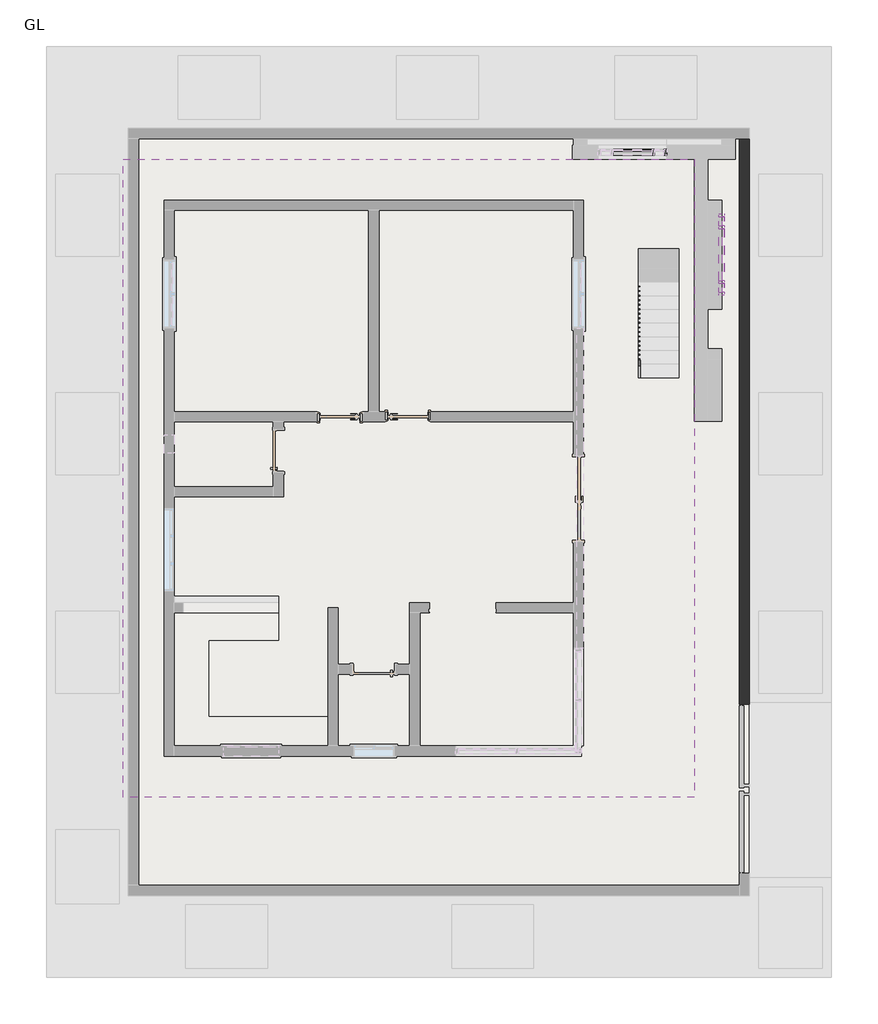
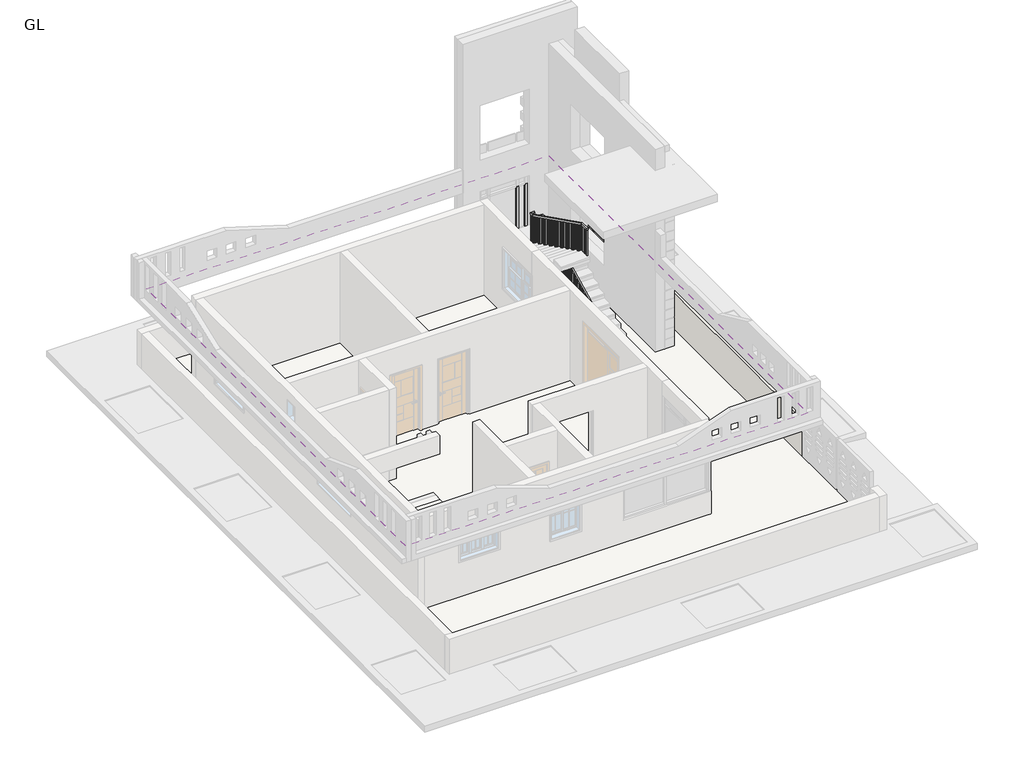
# One storey, part 3 of 4: 13 members, 3 plates, 2 slabs, 1 railing, 1 roof, 1 wall.
"""IFC4 building model written with IfcOpenShell, lengths in millimetres."""

from ifc_helpers import new_model, si_unit, frame, origin, origin_with_axes, place, context, project, spatial, polyline, outline, extrude, faceted_brep, transform, mapped, element, save
from components import member_e8ffc670, member_0c289f97, member_3782c11a, member_285512ba, member_6b401d40, member_96c05505, member_4491d118, member_82905deb, system_panel_glazed_d23cfa45, system_panel_glazed_ccd8c114, system_panel_glazed_e991d7fc

model = new_model("IFC4")

# Units and contexts
model_context = context("Model", 3, world=origin())
ifc_project = project(units=[si_unit("LENGTHUNIT", "METRE", prefix="MILLI")], contexts=[model_context])

# Site, building, storey
site = spatial("IfcSite", under=ifc_project)
building = spatial("IfcBuilding", under=site)
storey = spatial("IfcBuildingStorey", under=building, Name="GL", Elevation=0.0)

# Members
placement = place(None, origin())
member_shape = member_e8ffc670(model_context)
element("IfcMember", 1, ObjectType="Rectangular Mullion : 2.5\" x 5\" rectangular", at=placement, inside=storey, context=model_context, shape_type="MappedRepresentation", body=[
    mapped(member_shape, transform((872.7722402, 10698.1342801, 2741.3131867), x_axis=(0.0, 0.0, 1.0), y_axis=(1.0, 0.0, 0.0), z_axis=(0.0, 1.0, 0.0))),
])
member_2_shape = member_0c289f97(model_context)
element("IfcMember", 2, ObjectType="Rectangular Mullion : 2.5\" x 5\" rectangular", at=placement, inside=storey, context=model_context, shape_type="MappedRepresentation", body=[
    mapped(member_2_shape, transform((872.7722402, 8943.6292801, 2741.3131867), x_axis=(0.0, -1.0, 0.0), y_axis=(1.0, 0.0, 0.0), z_axis=(0.0, 0.0, 1.0))),
])
member_3_shape = member_3782c11a(model_context)
element("IfcMember", 3, ObjectType="Rectangular Mullion : 2.5\" x 5\" rectangular", at=placement, inside=storey, context=model_context, shape_type="MappedRepresentation", body=[
    mapped(member_3_shape, transform((872.7722402, 9007.1292801, 1219.2), x_axis=(0.0, 0.0, -1.0), y_axis=(1.0, 0.0, 0.0), z_axis=(0.0, -1.0, 0.0))),
])
element("IfcMember", 4, ObjectType="Rectangular Mullion : 2.5\" x 5\" rectangular", at=placement, inside=storey, context=model_context, shape_type="MappedRepresentation", body=[
    mapped(member_2_shape, transform((872.7722402, 10761.6342801, 1219.2), x_axis=(0.0, 1.0, 0.0), y_axis=(1.0, 0.0, 0.0), z_axis=(0.0, 0.0, -1.0))),
])
member_4_shape = member_285512ba(model_context)
element("IfcMember", 5, ObjectType="Rectangular Mullion : 2.5\" x 5\" rectangular", at=placement, inside=storey, context=model_context, shape_type="MappedRepresentation", body=[
    mapped(member_4_shape, transform((872.7722402, 9237.6342801, 2741.3131867), x_axis=(0.0, -1.0, 0.0), y_axis=(1.0, 0.0, 0.0), z_axis=(0.0, 0.0, 1.0))),
])
element("IfcMember", 6, ObjectType="Rectangular Mullion : 2.5\" x 5\" rectangular", at=placement, inside=storey, context=model_context, shape_type="MappedRepresentation", body=[
    mapped(member_4_shape, transform((872.7722402, 10461.9142801, 2741.3131867), x_axis=(0.0, -1.0, 0.0), y_axis=(1.0, 0.0, 0.0), z_axis=(0.0, 0.0, 1.0))),
])
member_5_shape = member_6b401d40(model_context)
element("IfcMember", 7, ObjectType="Rectangular Mullion : 2.5\" x 5\" rectangular", at=placement, inside=storey, context=model_context, shape_type="MappedRepresentation", body=[
    mapped(member_5_shape, transform((872.7722402, 10430.1642801, 2741.3131867), x_axis=(0.0, 0.0, 1.0), y_axis=(1.0, 0.0, 0.0), z_axis=(0.0, 1.0, 0.0))),
])
element("IfcMember", 8, ObjectType="Rectangular Mullion : 2.5\" x 5\" rectangular", at=placement, inside=storey, context=model_context, shape_type="MappedRepresentation", body=[
    mapped(member_5_shape, transform((872.7722402, 9269.3842801, 1219.2), x_axis=(0.0, 0.0, -1.0), y_axis=(1.0, 0.0, 0.0), z_axis=(0.0, -1.0, 0.0))),
])
element("IfcMember", 9, ObjectType="Rectangular Mullion : 2.5\" x 5\" rectangular", at=placement, inside=storey, context=model_context, shape_type="MappedRepresentation", body=[
    mapped(member_3_shape, transform((872.7722402, 9205.8842801, 2741.3131867), x_axis=(0.0, 0.0, 1.0), y_axis=(1.0, 0.0, 0.0), z_axis=(0.0, 1.0, 0.0))),
])
element("IfcMember", 10, ObjectType="Rectangular Mullion : 2.5\" x 5\" rectangular", at=placement, inside=storey, context=model_context, shape_type="MappedRepresentation", body=[
    mapped(member_shape, transform((872.7722402, 10493.6642801, 1219.2), x_axis=(0.0, 0.0, -1.0), y_axis=(1.0, 0.0, 0.0), z_axis=(0.0, -1.0, 0.0))),
])
member_6_shape = member_96c05505(model_context)
element("IfcMember", 11, ObjectType="Rectangular Mullion : 2.5\" x 5\" rectangular", at=placement, inside=storey, context=model_context, shape_type="MappedRepresentation", body=[
    mapped(member_6_shape, transform((-691.0183629, 12133.2342801, 767.08), x_axis=(0.0, 0.0, -1.0), y_axis=(0.0, 1.0, 0.0), z_axis=(1.0, 0.0, 0.0))),
])
member_7_shape = member_4491d118(model_context)
element("IfcMember", 12, ObjectType="Rectangular Mullion : 2.5\" x 5\" rectangular", at=placement, inside=storey, context=model_context, shape_type="MappedRepresentation", body=[
    mapped(member_7_shape, transform((-354.4683629, 12133.2342801, 2291.08), x_axis=(1.0, 0.0, 0.0), y_axis=(0.0, 1.0, 0.0), z_axis=(0.0, 0.0, 1.0))),
])
member_8_shape = member_82905deb(model_context)
element("IfcMember", 13, ObjectType="Rectangular Mullion : 2.5\" x 5\" rectangular", at=placement, inside=storey, context=model_context, shape_type="MappedRepresentation", body=[
    mapped(member_8_shape, transform((-659.2683629, 12133.2342801, 2291.08), x_axis=(1.0, 0.0, 0.0), y_axis=(0.0, 1.0, 0.0), z_axis=(0.0, 0.0, 1.0))),
])

# Plates
system_panel_glazed_shape = system_panel_glazed_d23cfa45(model_context)
element("IfcPlate", 14, ObjectType="System Panel : Glazed", at=placement, inside=storey, context=model_context, shape_type="MappedRepresentation", body=[
    mapped(system_panel_glazed_shape, transform((872.7722402, 10595.8992801, 1282.7), x_axis=(0.0, -1.0, 0.0), y_axis=(1.0, 0.0, 0.0), z_axis=(0.0, 0.0, 1.0))),
])
system_panel_glazed_2_shape = system_panel_glazed_ccd8c114(model_context)
element("IfcPlate", 15, ObjectType="System Panel : Glazed", at=placement, inside=storey, context=model_context, shape_type="MappedRepresentation", body=[
    mapped(system_panel_glazed_2_shape, transform((872.7722402, 9106.5067801, 1282.7), x_axis=(0.0, -1.0, 0.0), y_axis=(1.0, 0.0, 0.0), z_axis=(0.0, 0.0, 1.0))),
])
system_panel_glazed_3_shape = system_panel_glazed_e991d7fc(model_context)
element("IfcPlate", 16, ObjectType="System Panel : Glazed", at=placement, inside=storey, context=model_context, shape_type="MappedRepresentation", body=[
    mapped(system_panel_glazed_3_shape, transform((872.7722402, 9849.7742801, 1282.7), x_axis=(0.0, -1.0, 0.0), y_axis=(1.0, 0.0, 0.0), z_axis=(0.0, 0.0, 1.0))),
])

# Railing
element("IfcRailing", 17, ObjectType="Handrail - Rectangular", at=placement, inside=storey, context=model_context, shape_type="SolidModel", body=[
    faceted_brep([(-994.1277598, 7104.0342801, 1066.8), (-994.1277598, 7104.0342801, 1010.0038734), (-943.3277598, 7104.0342801, 1010.0038734), (-943.3277598, 7104.0342801, 1066.8), (-994.1277598, 10075.8342801, 2552.7), (-994.1277598, 10126.6342801, 2521.3038734), (-943.3277598, 10126.6342801, 2521.3038734), (-943.3277598, 10075.8342801, 2552.7), (-994.1277598, 10075.8342801, 2590.8), (-994.1277598, 10126.6342801, 2540.0), (-943.3277598, 10126.6342801, 2540.0), (-943.3277598, 10075.8342801, 2590.8), (-994.1277598, 10152.0342801, 2590.8), (-994.1277598, 10152.0342801, 2540.0), (-943.3277598, 10202.8342801, 2540.0), (-943.3277598, 10202.8342801, 2590.8), (-1070.3277598, 10152.0342801, 2590.8), (-1070.3277598, 10152.0342801, 2540.0), (-1070.3277598, 10202.8342801, 2540.0), (-1070.3277598, 10202.8342801, 2590.8), (-1222.7277598, 10152.0342801, 2590.8), (-1273.5277598, 10152.0342801, 2540.0), (-1273.5277598, 10202.8342801, 2540.0), (-1222.7277598, 10202.8342801, 2590.8), (-1222.7277598, 10152.0342801, 2781.3), (-1273.5277598, 10152.0342801, 2730.5), (-1273.5277598, 10202.8342801, 2730.5), (-1222.7277598, 10202.8342801, 2781.3), (-1298.9277598, 10152.0342801, 2781.3), (-1298.9277598, 10152.0342801, 2730.5), (-1349.7277598, 10202.8342801, 2730.5), (-1349.7277598, 10202.8342801, 2781.3), (-1298.9277598, 10075.8342801, 2781.3), (-1298.9277598, 10063.8420269, 2730.5), (-1349.7277598, 10063.8420269, 2730.5), (-1349.7277598, 10075.8342801, 2781.3), (-1298.9277598, 7408.8342801, 4114.8), (-1298.9277598, 7396.8420269, 4064.0), (-1349.7277598, 7396.8420269, 4064.0), (-1349.7277598, 7408.8342801, 4114.8), (-1298.9277598, 7104.0342801, 4114.8), (-1349.7277598, 7104.0342801, 4114.8), (-1349.7277598, 7104.0342801, 4064.0), (-1298.9277598, 7104.0342801, 4064.0)], [[[0, 1, 2, 3]], [[1, 0, 4, 5]], [[2, 1, 5, 6]], [[3, 2, 6, 7]], [[0, 3, 7, 4]], [[5, 4, 8, 9]], [[6, 5, 9, 10]], [[7, 6, 10, 11]], [[4, 7, 11, 8]], [[9, 8, 12, 13]], [[10, 9, 13, 14]], [[11, 10, 14, 15]], [[8, 11, 15, 12]], [[13, 12, 16, 17]], [[14, 13, 17, 18]], [[15, 14, 18, 19]], [[12, 15, 19, 16]], [[17, 16, 20, 21]], [[18, 17, 21, 22]], [[19, 18, 22, 23]], [[16, 19, 23, 20]], [[21, 20, 24, 25]], [[22, 21, 25, 26]], [[23, 22, 26, 27]], [[20, 23, 27, 24]], [[25, 24, 28, 29]], [[26, 25, 29, 30]], [[27, 26, 30, 31]], [[24, 27, 31, 28]], [[29, 28, 32, 33]], [[30, 29, 33, 34]], [[31, 30, 34, 35]], [[28, 31, 35, 32]], [[33, 32, 36, 37]], [[34, 33, 37, 38]], [[35, 34, 38, 39]], [[32, 35, 39, 36]], [[40, 41, 42, 43]], [[37, 36, 40, 43]], [[38, 37, 43, 42]], [[39, 38, 42, 41]], [[36, 39, 41, 40]]]),
    extrude(outline(polyline([(-1314.8027598, 7138.9592801), (-1314.8027598, 7119.9092801), (-1333.8527598, 7119.9092801), (-1333.8527598, 7138.9592801), (-1314.8027598, 7138.9592801)])), frame((0.0, 0.0, 3200.4), z_axis=(0.0, 0.0, 1.0), x_axis=(1.0, 0.0, 0.0)), (0.0, 0.0, 1.0), 863.6),
    extrude(outline(polyline([(-1314.8027598, 7240.5592801), (-1314.8027598, 7221.5092801), (-1333.8527598, 7221.5092801), (-1333.8527598, 7240.5592801), (-1314.8027598, 7240.5592801)])), frame((0.0, 0.0, 3200.4), z_axis=(0.0, 0.0, 1.0), x_axis=(1.0, 0.0, 0.0)), (0.0, 0.0, 1.0), 863.6),
    extrude(outline(polyline([(-1314.8027598, 7342.1592801), (-1314.8027598, 7323.1092801), (-1333.8527598, 7323.1092801), (-1333.8527598, 7342.1592801), (-1314.8027598, 7342.1592801)])), frame((0.0, 0.0, 3200.4), z_axis=(0.0, 0.0, 1.0), x_axis=(1.0, 0.0, 0.0)), (0.0, 0.0, 1.0), 863.6),
    extrude(outline(polyline([(7443.7592801, 4040.5413734), (7443.7592801, 3048.0), (7424.7092801, 3048.0), (7424.7092801, 4050.0663734), (7443.7592801, 4040.5413734)])), frame((-1333.8527598, 0.0, 0.0), z_axis=(1.0, 0.0, 0.0), x_axis=(0.0, 1.0, 0.0)), (0.0, 0.0, 1.0), 19.05),
    extrude(outline(polyline([(7545.3592801, 3989.7413734), (7545.3592801, 3048.0), (7526.3092801, 3048.0), (7526.3092801, 3999.2663734), (7545.3592801, 3989.7413734)])), frame((-1333.8527598, 0.0, 0.0), z_axis=(1.0, 0.0, 0.0), x_axis=(0.0, 1.0, 0.0)), (0.0, 0.0, 1.0), 19.05),
    extrude(outline(polyline([(7646.9592801, 3938.9413734), (7646.9592801, 3048.0), (7627.9092801, 3048.0), (7627.9092801, 3948.4663734), (7646.9592801, 3938.9413734)])), frame((-1333.8527598, 0.0, 0.0), z_axis=(1.0, 0.0, 0.0), x_axis=(0.0, 1.0, 0.0)), (0.0, 0.0, 1.0), 19.05),
    extrude(outline(polyline([(7748.5592801, 3888.1413734), (7748.5592801, 2895.6), (7729.5092801, 2895.6), (7729.5092801, 3897.6663734), (7748.5592801, 3888.1413734)])), frame((-1333.8527598, 0.0, 0.0), z_axis=(1.0, 0.0, 0.0), x_axis=(0.0, 1.0, 0.0)), (0.0, 0.0, 1.0), 19.05),
    extrude(outline(polyline([(7850.1592801, 3837.3413734), (7850.1592801, 2895.6), (7831.1092801, 2895.6), (7831.1092801, 3846.8663734), (7850.1592801, 3837.3413734)])), frame((-1333.8527598, 0.0, 0.0), z_axis=(1.0, 0.0, 0.0), x_axis=(0.0, 1.0, 0.0)), (0.0, 0.0, 1.0), 19.05),
    extrude(outline(polyline([(7951.7592801, 3786.5413734), (7951.7592801, 2895.6), (7932.7092801, 2895.6), (7932.7092801, 3796.0663734), (7951.7592801, 3786.5413734)])), frame((-1333.8527598, 0.0, 0.0), z_axis=(1.0, 0.0, 0.0), x_axis=(0.0, 1.0, 0.0)), (0.0, 0.0, 1.0), 19.05),
    extrude(outline(polyline([(8053.3592801, 3735.7413734), (8053.3592801, 2743.2), (8034.3092801, 2743.2), (8034.3092801, 3745.2663734), (8053.3592801, 3735.7413734)])), frame((-1333.8527598, 0.0, 0.0), z_axis=(1.0, 0.0, 0.0), x_axis=(0.0, 1.0, 0.0)), (0.0, 0.0, 1.0), 19.05),
    extrude(outline(polyline([(8154.9592801, 3684.9413734), (8154.9592801, 2743.2), (8135.9092801, 2743.2), (8135.9092801, 3694.4663734), (8154.9592801, 3684.9413734)])), frame((-1333.8527598, 0.0, 0.0), z_axis=(1.0, 0.0, 0.0), x_axis=(0.0, 1.0, 0.0)), (0.0, 0.0, 1.0), 19.05),
    extrude(outline(polyline([(8256.5592801, 3634.1413734), (8256.5592801, 2743.2), (8237.5092801, 2743.2), (8237.5092801, 3643.6663734), (8256.5592801, 3634.1413734)])), frame((-1333.8527598, 0.0, 0.0), z_axis=(1.0, 0.0, 0.0), x_axis=(0.0, 1.0, 0.0)), (0.0, 0.0, 1.0), 19.05),
    extrude(outline(polyline([(8358.1592801, 3583.3413734), (8358.1592801, 2590.8), (8339.1092801, 2590.8), (8339.1092801, 3592.8663734), (8358.1592801, 3583.3413734)])), frame((-1333.8527598, 0.0, 0.0), z_axis=(1.0, 0.0, 0.0), x_axis=(0.0, 1.0, 0.0)), (0.0, 0.0, 1.0), 19.05),
    extrude(outline(polyline([(8459.7592801, 3532.5413734), (8459.7592801, 2590.8), (8440.7092801, 2590.8), (8440.7092801, 3542.0663734), (8459.7592801, 3532.5413734)])), frame((-1333.8527598, 0.0, 0.0), z_axis=(1.0, 0.0, 0.0), x_axis=(0.0, 1.0, 0.0)), (0.0, 0.0, 1.0), 19.05),
    extrude(outline(polyline([(8561.3592801, 3481.7413734), (8561.3592801, 2590.8), (8542.3092801, 2590.8), (8542.3092801, 3491.2663734), (8561.3592801, 3481.7413734)])), frame((-1333.8527598, 0.0, 0.0), z_axis=(1.0, 0.0, 0.0), x_axis=(0.0, 1.0, 0.0)), (0.0, 0.0, 1.0), 19.05),
    extrude(outline(polyline([(8662.9592801, 3430.9413734), (8662.9592801, 2438.4), (8643.9092801, 2438.4), (8643.9092801, 3440.4663734), (8662.9592801, 3430.9413734)])), frame((-1333.8527598, 0.0, 0.0), z_axis=(1.0, 0.0, 0.0), x_axis=(0.0, 1.0, 0.0)), (0.0, 0.0, 1.0), 19.05),
    extrude(outline(polyline([(8764.5592801, 3380.1413734), (8764.5592801, 2438.4), (8745.5092801, 2438.4), (8745.5092801, 3389.6663734), (8764.5592801, 3380.1413734)])), frame((-1333.8527598, 0.0, 0.0), z_axis=(1.0, 0.0, 0.0), x_axis=(0.0, 1.0, 0.0)), (0.0, 0.0, 1.0), 19.05),
    extrude(outline(polyline([(8866.1592801, 3329.3413734), (8866.1592801, 2438.4), (8847.1092801, 2438.4), (8847.1092801, 3338.8663734), (8866.1592801, 3329.3413734)])), frame((-1333.8527598, 0.0, 0.0), z_axis=(1.0, 0.0, 0.0), x_axis=(0.0, 1.0, 0.0)), (0.0, 0.0, 1.0), 19.05),
    extrude(outline(polyline([(8967.7592801, 3278.5413734), (8967.7592801, 2286.0), (8948.7092801, 2286.0), (8948.7092801, 3288.0663734), (8967.7592801, 3278.5413734)])), frame((-1333.8527598, 0.0, 0.0), z_axis=(1.0, 0.0, 0.0), x_axis=(0.0, 1.0, 0.0)), (0.0, 0.0, 1.0), 19.05),
    extrude(outline(polyline([(9069.3592801, 3227.7413734), (9069.3592801, 2286.0), (9050.3092801, 2286.0), (9050.3092801, 3237.2663734), (9069.3592801, 3227.7413734)])), frame((-1333.8527598, 0.0, 0.0), z_axis=(1.0, 0.0, 0.0), x_axis=(0.0, 1.0, 0.0)), (0.0, 0.0, 1.0), 19.05),
    extrude(outline(polyline([(9170.9592801, 3176.9413734), (9170.9592801, 2286.0), (9151.9092801, 2286.0), (9151.9092801, 3186.4663734), (9170.9592801, 3176.9413734)])), frame((-1333.8527598, 0.0, 0.0), z_axis=(1.0, 0.0, 0.0), x_axis=(0.0, 1.0, 0.0)), (0.0, 0.0, 1.0), 19.05),
    extrude(outline(polyline([(9272.5592801, 3126.1413734), (9272.5592801, 2133.6), (9253.5092801, 2133.6), (9253.5092801, 3135.6663734), (9272.5592801, 3126.1413734)])), frame((-1333.8527598, 0.0, 0.0), z_axis=(1.0, 0.0, 0.0), x_axis=(0.0, 1.0, 0.0)), (0.0, 0.0, 1.0), 19.05),
    extrude(outline(polyline([(9374.1592801, 3075.3413734), (9374.1592801, 2133.6), (9355.1092801, 2133.6), (9355.1092801, 3084.8663734), (9374.1592801, 3075.3413734)])), frame((-1333.8527598, 0.0, 0.0), z_axis=(1.0, 0.0, 0.0), x_axis=(0.0, 1.0, 0.0)), (0.0, 0.0, 1.0), 19.05),
    extrude(outline(polyline([(9475.7592801, 3024.5413734), (9475.7592801, 2133.6), (9456.7092801, 2133.6), (9456.7092801, 3034.0663734), (9475.7592801, 3024.5413734)])), frame((-1333.8527598, 0.0, 0.0), z_axis=(1.0, 0.0, 0.0), x_axis=(0.0, 1.0, 0.0)), (0.0, 0.0, 1.0), 19.05),
    extrude(outline(polyline([(9577.3592801, 2973.7413734), (9577.3592801, 1981.2), (9558.3092801, 1981.2), (9558.3092801, 2983.2663734), (9577.3592801, 2973.7413734)])), frame((-1333.8527598, 0.0, 0.0), z_axis=(1.0, 0.0, 0.0), x_axis=(0.0, 1.0, 0.0)), (0.0, 0.0, 1.0), 19.05),
    extrude(outline(polyline([(9678.9592801, 2922.9413734), (9678.9592801, 1981.2), (9659.9092801, 1981.2), (9659.9092801, 2932.4663734), (9678.9592801, 2922.9413734)])), frame((-1333.8527598, 0.0, 0.0), z_axis=(1.0, 0.0, 0.0), x_axis=(0.0, 1.0, 0.0)), (0.0, 0.0, 1.0), 19.05),
    extrude(outline(polyline([(9780.5592801, 2872.1413734), (9780.5592801, 1981.2), (9761.5092801, 1981.2), (9761.5092801, 2881.6663734), (9780.5592801, 2872.1413734)])), frame((-1333.8527598, 0.0, 0.0), z_axis=(1.0, 0.0, 0.0), x_axis=(0.0, 1.0, 0.0)), (0.0, 0.0, 1.0), 19.05),
    extrude(outline(polyline([(9882.1592801, 2821.3413734), (9882.1592801, 1828.8), (9863.1092801, 1828.8), (9863.1092801, 2830.8663734), (9882.1592801, 2821.3413734)])), frame((-1333.8527598, 0.0, 0.0), z_axis=(1.0, 0.0, 0.0), x_axis=(0.0, 1.0, 0.0)), (0.0, 0.0, 1.0), 19.05),
    extrude(outline(polyline([(9983.7592801, 2770.5413734), (9983.7592801, 1828.8), (9964.7092801, 1828.8), (9964.7092801, 2780.0663734), (9983.7592801, 2770.5413734)])), frame((-1333.8527598, 0.0, 0.0), z_axis=(1.0, 0.0, 0.0), x_axis=(0.0, 1.0, 0.0)), (0.0, 0.0, 1.0), 19.05),
    extrude(outline(polyline([(10085.3592801, 2719.7413734), (10085.3592801, 1828.8), (10066.3092801, 1828.8), (10066.3092801, 2729.2663734), (10085.3592801, 2719.7413734)])), frame((-1333.8527598, 0.0, 0.0), z_axis=(1.0, 0.0, 0.0), x_axis=(0.0, 1.0, 0.0)), (0.0, 0.0, 1.0), 19.05),
    extrude(outline(polyline([(-1264.0027598, 10167.9092801), (-1283.0527598, 10167.9092801), (-1283.0527598, 10186.9592801), (-1264.0027598, 10186.9592801), (-1264.0027598, 10167.9092801)])), frame((0.0, 0.0, 1676.4), z_axis=(0.0, 0.0, 1.0), x_axis=(1.0, 0.0, 0.0)), (0.0, 0.0, 1.0), 1054.1),
    extrude(outline(polyline([(-1162.4027598, 10167.9092801), (-1181.4527598, 10167.9092801), (-1181.4527598, 10186.9592801), (-1162.4027598, 10186.9592801), (-1162.4027598, 10167.9092801)])), frame((0.0, 0.0, 1676.4), z_axis=(0.0, 0.0, 1.0), x_axis=(1.0, 0.0, 0.0)), (0.0, 0.0, 1.0), 863.6),
    extrude(outline(polyline([(-1060.8027598, 10167.9092801), (-1079.8527598, 10167.9092801), (-1079.8527598, 10186.9592801), (-1060.8027598, 10186.9592801), (-1060.8027598, 10167.9092801)])), frame((0.0, 0.0, 1676.4), z_axis=(0.0, 0.0, 1.0), x_axis=(1.0, 0.0, 0.0)), (0.0, 0.0, 1.0), 863.6),
    extrude(outline(polyline([(-978.2527598, 10142.5092801), (-978.2527598, 10161.5592801), (-959.2027598, 10161.5592801), (-959.2027598, 10142.5092801), (-978.2527598, 10142.5092801)])), frame((0.0, 0.0, 1676.4), z_axis=(0.0, 0.0, 1.0), x_axis=(1.0, 0.0, 0.0)), (0.0, 0.0, 1.0), 863.6),
    extrude(outline(polyline([(10059.9592801, 2487.9663734), (10059.9592801, 1524.0), (10040.9092801, 1524.0), (10040.9092801, 2478.4413734), (10059.9592801, 2487.9663734)])), frame((-978.2527598, 0.0, 0.0), z_axis=(1.0, 0.0, 0.0), x_axis=(0.0, 1.0, 0.0)), (0.0, 0.0, 1.0), 19.05),
    extrude(outline(polyline([(9958.3592801, 2437.1663734), (9958.3592801, 1524.0), (9939.3092801, 1524.0), (9939.3092801, 2427.6413734), (9958.3592801, 2437.1663734)])), frame((-978.2527598, 0.0, 0.0), z_axis=(1.0, 0.0, 0.0), x_axis=(0.0, 1.0, 0.0)), (0.0, 0.0, 1.0), 19.05),
    extrude(outline(polyline([(9856.7592801, 2386.3663734), (9856.7592801, 1524.0), (9837.7092801, 1524.0), (9837.7092801, 2376.8413734), (9856.7592801, 2386.3663734)])), frame((-978.2527598, 0.0, 0.0), z_axis=(1.0, 0.0, 0.0), x_axis=(0.0, 1.0, 0.0)), (0.0, 0.0, 1.0), 19.05),
    extrude(outline(polyline([(9755.1592801, 2335.5663734), (9755.1592801, 1371.6), (9736.1092801, 1371.6), (9736.1092801, 2326.0413734), (9755.1592801, 2335.5663734)])), frame((-978.2527598, 0.0, 0.0), z_axis=(1.0, 0.0, 0.0), x_axis=(0.0, 1.0, 0.0)), (0.0, 0.0, 1.0), 19.05),
    extrude(outline(polyline([(9653.5592801, 2284.7663734), (9653.5592801, 1371.6), (9634.5092801, 1371.6), (9634.5092801, 2275.2413734), (9653.5592801, 2284.7663734)])), frame((-978.2527598, 0.0, 0.0), z_axis=(1.0, 0.0, 0.0), x_axis=(0.0, 1.0, 0.0)), (0.0, 0.0, 1.0), 19.05),
    extrude(outline(polyline([(9551.9592801, 2233.9663734), (9551.9592801, 1371.6), (9532.9092801, 1371.6), (9532.9092801, 2224.4413734), (9551.9592801, 2233.9663734)])), frame((-978.2527598, 0.0, 0.0), z_axis=(1.0, 0.0, 0.0), x_axis=(0.0, 1.0, 0.0)), (0.0, 0.0, 1.0), 19.05),
    extrude(outline(polyline([(9450.3592801, 2183.1663734), (9450.3592801, 1219.2), (9431.3092801, 1219.2), (9431.3092801, 2173.6413734), (9450.3592801, 2183.1663734)])), frame((-978.2527598, 0.0, 0.0), z_axis=(1.0, 0.0, 0.0), x_axis=(0.0, 1.0, 0.0)), (0.0, 0.0, 1.0), 19.05),
    extrude(outline(polyline([(9348.7592801, 2132.3663734), (9348.7592801, 1219.2), (9329.7092801, 1219.2), (9329.7092801, 2122.8413734), (9348.7592801, 2132.3663734)])), frame((-978.2527598, 0.0, 0.0), z_axis=(1.0, 0.0, 0.0), x_axis=(0.0, 1.0, 0.0)), (0.0, 0.0, 1.0), 19.05),
    extrude(outline(polyline([(9247.1592801, 2081.5663734), (9247.1592801, 1219.2), (9228.1092801, 1219.2), (9228.1092801, 2072.0413734), (9247.1592801, 2081.5663734)])), frame((-978.2527598, 0.0, 0.0), z_axis=(1.0, 0.0, 0.0), x_axis=(0.0, 1.0, 0.0)), (0.0, 0.0, 1.0), 19.05),
    extrude(outline(polyline([(9145.5592801, 2030.7663734), (9145.5592801, 1066.8), (9126.5092801, 1066.8), (9126.5092801, 2021.2413734), (9145.5592801, 2030.7663734)])), frame((-978.2527598, 0.0, 0.0), z_axis=(1.0, 0.0, 0.0), x_axis=(0.0, 1.0, 0.0)), (0.0, 0.0, 1.0), 19.05),
    extrude(outline(polyline([(9043.9592801, 1979.9663734), (9043.9592801, 1066.8), (9024.9092801, 1066.8), (9024.9092801, 1970.4413734), (9043.9592801, 1979.9663734)])), frame((-978.2527598, 0.0, 0.0), z_axis=(1.0, 0.0, 0.0), x_axis=(0.0, 1.0, 0.0)), (0.0, 0.0, 1.0), 19.05),
    extrude(outline(polyline([(8942.3592801, 1929.1663734), (8942.3592801, 1066.8), (8923.3092801, 1066.8), (8923.3092801, 1919.6413734), (8942.3592801, 1929.1663734)])), frame((-978.2527598, 0.0, 0.0), z_axis=(1.0, 0.0, 0.0), x_axis=(0.0, 1.0, 0.0)), (0.0, 0.0, 1.0), 19.05),
    extrude(outline(polyline([(8840.7592801, 1878.3663734), (8840.7592801, 914.4), (8821.7092801, 914.4), (8821.7092801, 1868.8413734), (8840.7592801, 1878.3663734)])), frame((-978.2527598, 0.0, 0.0), z_axis=(1.0, 0.0, 0.0), x_axis=(0.0, 1.0, 0.0)), (0.0, 0.0, 1.0), 19.05),
    extrude(outline(polyline([(8739.1592801, 1827.5663734), (8739.1592801, 914.4), (8720.1092801, 914.4), (8720.1092801, 1818.0413734), (8739.1592801, 1827.5663734)])), frame((-978.2527598, 0.0, 0.0), z_axis=(1.0, 0.0, 0.0), x_axis=(0.0, 1.0, 0.0)), (0.0, 0.0, 1.0), 19.05),
    extrude(outline(polyline([(8637.5592801, 1776.7663734), (8637.5592801, 914.4), (8618.5092801, 914.4), (8618.5092801, 1767.2413734), (8637.5592801, 1776.7663734)])), frame((-978.2527598, 0.0, 0.0), z_axis=(1.0, 0.0, 0.0), x_axis=(0.0, 1.0, 0.0)), (0.0, 0.0, 1.0), 19.05),
    extrude(outline(polyline([(8535.9592801, 1725.9663734), (8535.9592801, 762.0), (8516.9092801, 762.0), (8516.9092801, 1716.4413734), (8535.9592801, 1725.9663734)])), frame((-978.2527598, 0.0, 0.0), z_axis=(1.0, 0.0, 0.0), x_axis=(0.0, 1.0, 0.0)), (0.0, 0.0, 1.0), 19.05),
    extrude(outline(polyline([(8434.3592801, 1675.1663734), (8434.3592801, 762.0), (8415.3092801, 762.0), (8415.3092801, 1665.6413734), (8434.3592801, 1675.1663734)])), frame((-978.2527598, 0.0, 0.0), z_axis=(1.0, 0.0, 0.0), x_axis=(0.0, 1.0, 0.0)), (0.0, 0.0, 1.0), 19.05),
    extrude(outline(polyline([(8332.7592801, 1624.3663734), (8332.7592801, 762.0), (8313.7092801, 762.0), (8313.7092801, 1614.8413734), (8332.7592801, 1624.3663734)])), frame((-978.2527598, 0.0, 0.0), z_axis=(1.0, 0.0, 0.0), x_axis=(0.0, 1.0, 0.0)), (0.0, 0.0, 1.0), 19.05),
    extrude(outline(polyline([(8231.1592801, 1573.5663734), (8231.1592801, 609.6), (8212.1092801, 609.6), (8212.1092801, 1564.0413734), (8231.1592801, 1573.5663734)])), frame((-978.2527598, 0.0, 0.0), z_axis=(1.0, 0.0, 0.0), x_axis=(0.0, 1.0, 0.0)), (0.0, 0.0, 1.0), 19.05),
    extrude(outline(polyline([(8129.5592801, 1522.7663734), (8129.5592801, 609.6), (8110.5092801, 609.6), (8110.5092801, 1513.2413734), (8129.5592801, 1522.7663734)])), frame((-978.2527598, 0.0, 0.0), z_axis=(1.0, 0.0, 0.0), x_axis=(0.0, 1.0, 0.0)), (0.0, 0.0, 1.0), 19.05),
    extrude(outline(polyline([(8027.9592801, 1471.9663734), (8027.9592801, 609.6), (8008.9092801, 609.6), (8008.9092801, 1462.4413734), (8027.9592801, 1471.9663734)])), frame((-978.2527598, 0.0, 0.0), z_axis=(1.0, 0.0, 0.0), x_axis=(0.0, 1.0, 0.0)), (0.0, 0.0, 1.0), 19.05),
    extrude(outline(polyline([(7926.3592801, 1421.1663734), (7926.3592801, 457.2), (7907.3092801, 457.2), (7907.3092801, 1411.6413734), (7926.3592801, 1421.1663734)])), frame((-978.2527598, 0.0, 0.0), z_axis=(1.0, 0.0, 0.0), x_axis=(0.0, 1.0, 0.0)), (0.0, 0.0, 1.0), 19.05),
    extrude(outline(polyline([(7824.7592801, 1370.3663734), (7824.7592801, 457.2), (7805.7092801, 457.2), (7805.7092801, 1360.8413734), (7824.7592801, 1370.3663734)])), frame((-978.2527598, 0.0, 0.0), z_axis=(1.0, 0.0, 0.0), x_axis=(0.0, 1.0, 0.0)), (0.0, 0.0, 1.0), 19.05),
    extrude(outline(polyline([(7723.1592801, 1319.5663734), (7723.1592801, 457.2), (7704.1092801, 457.2), (7704.1092801, 1310.0413734), (7723.1592801, 1319.5663734)])), frame((-978.2527598, 0.0, 0.0), z_axis=(1.0, 0.0, 0.0), x_axis=(0.0, 1.0, 0.0)), (0.0, 0.0, 1.0), 19.05),
    extrude(outline(polyline([(7621.5592801, 1268.7663734), (7621.5592801, 304.8), (7602.5092801, 304.8), (7602.5092801, 1259.2413734), (7621.5592801, 1268.7663734)])), frame((-978.2527598, 0.0, 0.0), z_axis=(1.0, 0.0, 0.0), x_axis=(0.0, 1.0, 0.0)), (0.0, 0.0, 1.0), 19.05),
    extrude(outline(polyline([(7519.9592801, 1217.9663734), (7519.9592801, 304.8), (7500.9092801, 304.8), (7500.9092801, 1208.4413734), (7519.9592801, 1217.9663734)])), frame((-978.2527598, 0.0, 0.0), z_axis=(1.0, 0.0, 0.0), x_axis=(0.0, 1.0, 0.0)), (0.0, 0.0, 1.0), 19.05),
    extrude(outline(polyline([(7418.3592801, 1167.1663734), (7418.3592801, 304.8), (7399.3092801, 304.8), (7399.3092801, 1157.6413734), (7418.3592801, 1167.1663734)])), frame((-978.2527598, 0.0, 0.0), z_axis=(1.0, 0.0, 0.0), x_axis=(0.0, 1.0, 0.0)), (0.0, 0.0, 1.0), 19.05),
    extrude(outline(polyline([(7316.7592801, 1116.3663734), (7316.7592801, 152.4), (7297.7092801, 152.4), (7297.7092801, 1106.8413734), (7316.7592801, 1116.3663734)])), frame((-978.2527598, 0.0, 0.0), z_axis=(1.0, 0.0, 0.0), x_axis=(0.0, 1.0, 0.0)), (0.0, 0.0, 1.0), 19.05),
    extrude(outline(polyline([(7215.1592801, 1065.5663734), (7215.1592801, 152.4), (7196.1092801, 152.4), (7196.1092801, 1056.0413734), (7215.1592801, 1065.5663734)])), frame((-978.2527598, 0.0, 0.0), z_axis=(1.0, 0.0, 0.0), x_axis=(0.0, 1.0, 0.0)), (0.0, 0.0, 1.0), 19.05),
    extrude(outline(polyline([(-1314.8027598, 10167.9092801), (-1333.8527598, 10167.9092801), (-1333.8527598, 10186.9592801), (-1314.8027598, 10186.9592801), (-1314.8027598, 10167.9092801)])), frame((0.0, 0.0, 1676.4), z_axis=(0.0, 0.0, 1.0), x_axis=(1.0, 0.0, 0.0)), (0.0, 0.0, 1.0), 1054.1),
    extrude(outline(polyline([(-978.2527598, 10167.9092801), (-978.2527598, 10186.9592801), (-959.2027598, 10186.9592801), (-959.2027598, 10167.9092801), (-978.2527598, 10167.9092801)])), frame((0.0, 0.0, 1676.4), z_axis=(0.0, 0.0, 1.0), x_axis=(1.0, 0.0, 0.0)), (0.0, 0.0, 1.0), 863.6),
    extrude(outline(polyline([(-1314.8027598, 7123.0842801), (-1314.8027598, 7104.0342801), (-1333.8527598, 7104.0342801), (-1333.8527598, 7123.0842801), (-1314.8027598, 7123.0842801)])), frame((0.0, 0.0, 3200.4), z_axis=(0.0, 0.0, 1.0), x_axis=(1.0, 0.0, 0.0)), (0.0, 0.0, 1.0), 863.6),
    extrude(outline(polyline([(7123.0842801, 1019.5288734), (7123.0842801, 152.4), (7104.0342801, 152.4), (7104.0342801, 1010.0038734), (7123.0842801, 1019.5288734)])), frame((-978.2527598, 0.0, 0.0), z_axis=(1.0, 0.0, 0.0), x_axis=(0.0, 1.0, 0.0)), (0.0, 0.0, 1.0), 19.05),
])

# Roof
element("IfcRoof", 18, ObjectType="Generic - 6\"", at=placement, inside=storey, context=model_context, shape_type="SweptSolid", body=[
    extrude(outline(polyline([(-12500.3277598, 11980.8342801), (263.1722402, 11980.8342801), (263.1722402, -2268.5657199), (-12500.3277598, -2268.5657199), (-12500.3277598, 11980.8342801)]), holes=[polyline([(-2213.3277598, 11066.4342801), (-2213.3277598, 7104.0342801), (34.5722402, 7104.0342801), (34.5722402, 11066.4342801), (-2213.3277598, 11066.4342801)])]), frame((0.0, 0.0, 3048.0), z_axis=(0.0, 0.0, 1.0), x_axis=(1.0, 0.0, 0.0)), (0.0, 0.0, 1.0), 152.4),
])

# Slabs
element("IfcSlab", 19, ObjectType="Generic - 6\"", at=placement, inside=storey, context=model_context, shape_type="SweptSolid", body=[
    extrude(outline(polyline([(1495.0722402, 12666.6342801), (1495.0722402, -4465.6657199), (-12386.0277598, -4465.6657199), (-12386.0277598, 12666.6342801), (1495.0722402, 12666.6342801)])), frame((0.0, 0.0, -152.4), z_axis=(0.0, 0.0, 1.0), x_axis=(1.0, 0.0, 0.0)), (0.0, 0.0, 1.0), 152.4),
])
element("IfcSlab", 20, ObjectType="Kitchen floor", at=placement, inside=storey, context=model_context, shape_type="SweptSolid", body=[
    extrude(outline(polyline([(-10595.3277598, 1236.6342801), (-10595.3277598, -477.8657199), (-7928.3277598, -477.8657199), (-7928.3277598, -1125.5657199), (-11357.3277598, -1125.5657199), (-11357.3277598, 1846.2342801), (-9033.2277598, 1846.2342801), (-9033.2277598, 1236.6342801), (-10595.3277598, 1236.6342801)])), frame((0.0, 0.0, 838.2), z_axis=(0.0, 0.0, 1.0), x_axis=(1.0, 0.0, 0.0)), (0.0, 0.0, 1.0), 76.2),
])

# Wall
element("IfcWall", 21, ObjectType="Generic - 9\"", at=placement, inside=storey, context=model_context, shape_type="SweptSolid", body=[
    extrude(outline(polyline([(1266.4722402, -198.4657199), (1266.4722402, 12438.0342801), (1495.0722402, 12438.0342801), (1495.0722402, -198.4657199), (1266.4722402, -198.4657199)])), origin_with_axes(), (0.0, 0.0, 1.0), 1219.2),
])

save(model, "model.ifc")

# Revit data of these elements
# Type "Rectangular Mullion : 2.5\" x 5\" rectangular"
#   built-in parameter 1007304 = 0.416667 (stored number, unit not read)
#   built-in parameter 1007301 = 0.104167 (stored number, unit not read)
#   built-in parameter 1007300 = 0.104167 (stored number, unit not read)
# Type "System Panel : Glazed"
#   Construction Type Id = "GSP4R"
#   Analytic Construction = "1/8 in Pilkington single glazing"
#   Visual Light Transmittance = 0.9
#   Solar Heat Gain Coefficient = 0.86
#   Heat Transfer Coefficient (U) = 1.18115 BTU/(h·ft²·°F)
#   Define Thermal Properties by = 1
# Type "Handrail - Rectangular"
#   built-in parameter 1008612 = 0.0416667 (stored number, unit not read)
#   built-in parameter 1008611 = 0.0416667 (stored number, unit not read)
#   built-in parameter 1008609 = 0.333333 (stored number, unit not read)
#   built-in parameter 1008604 = 0.166667 (stored number, unit not read)
#   built-in parameter 1008603 = 0.166667 (stored number, unit not read)
#   Railing Height = 3' - 0"
#   built-in parameter 1008630 = 2
#   built-in parameter 1008610 = 2
#   built-in parameter 1008618 = Baluster - Square : 3/4"
# Type "Generic - 6\""
#   Layers, outside or top first: 0' - 6" "Concrete, Precast" (function 1)
# Type "Generic - 6\""
#   Function = 0
#   Layers, outside or top first: 0' - 6" "Concrete, Cast-in-Place gray" (function 1)
# Type "Kitchen floor"
#   Function = 0
#   Layers, outside or top first: 0' - 3" "Kitchen floor" (function 1)
# Type "Generic - 9\""
#   Layers, outside or top first: 0' - 0 1/2" no material (function 4); 0' - 8" "Brick, Common" (function 1); 0' - 0 1/2" no material (function 5)
# Elements 1, 2, 3, 4, 5, 6, 7, 8, 9, 10, 11, 12, 13 (IfcMember, "Rectangular Mullion : 2.5\" x 5\" rectangular")
#   Phase Created = New Construction
#   Materials on its faces: "Aluminum"
# Elements 14, 15, 16 (IfcPlate, "System Panel : Glazed")
#   Phase Created = New Construction
#   Materials on its faces: "Glass"
# Element 17 (IfcRailing, "Handrail - Rectangular")
#   Phase Created = New Construction
# Element 18 (IfcRoof, "Generic - 6\"")
#   built-in parameter 1001705 = 10.5 (stored number, unit not read)
#   built-in parameter 1001701 = 10 (stored number, unit not read)
#   built-in parameter 1001710 = 33615
#   Phase Created = New Construction
#   Materials on its faces: "Concrete, Precast"
# Element 19 (IfcSlab, "Generic - 6\"")
#   Height Offset From Level = 0' - 0"
#   Phase Created = New Construction
#   Materials on its faces: "Concrete, Cast-in-Place gray"
# Element 20 (IfcSlab, "Kitchen floor")
#   built-in parameter 1001955 = 3.14159 (stored number, unit not read)
#   Height Offset From Level = 3' - 0"
#   Phase Created = New Construction
#   Materials on its faces: "Kitchen floor"
# Element 21 (IfcWall, "Generic - 9\"")
#   Top Offset = -0' - 6"
#   Base Offset = 0' - 0"
#   Unconnected Height = 4' - 0"
#   wall height = 4' - 0"
#   Phase Created = New Construction
#   Base Constraint = GL
#   Materials on its faces: "Default Wall"
# Materials
#   "Concrete, Precast": class "Concrete", colour RGB 130 132 119, transparency 0, Description = "Precast concrete", Cost = 0
#   "Concrete, Cast-in-Place gray": class "Concrete", colour RGB 130 132 119, transparency 0, Description = "Cast-in-place concrete", Cost = 0
#   "Kitchen floor": class "Generic", colour RGB 173 179 190, transparency 0, Cost = 0
#   "Brick, Common": class "Masonry", colour RGB 85 47 55, transparency 0, Description = "Common brick", Cost = 0
#   "Aluminum": class "Metal", colour RGB 247 247 247, transparency 0, Description = "Aluminum 6061", Cost = 0
#   "Glass": class "Glass", colour RGB 0 128 192, transparency 0.75, Description = "Soda Lime Glass", Cost = 0
#   "Default Wall": colour RGB 128 128 128, transparency 0, Cost = 0
